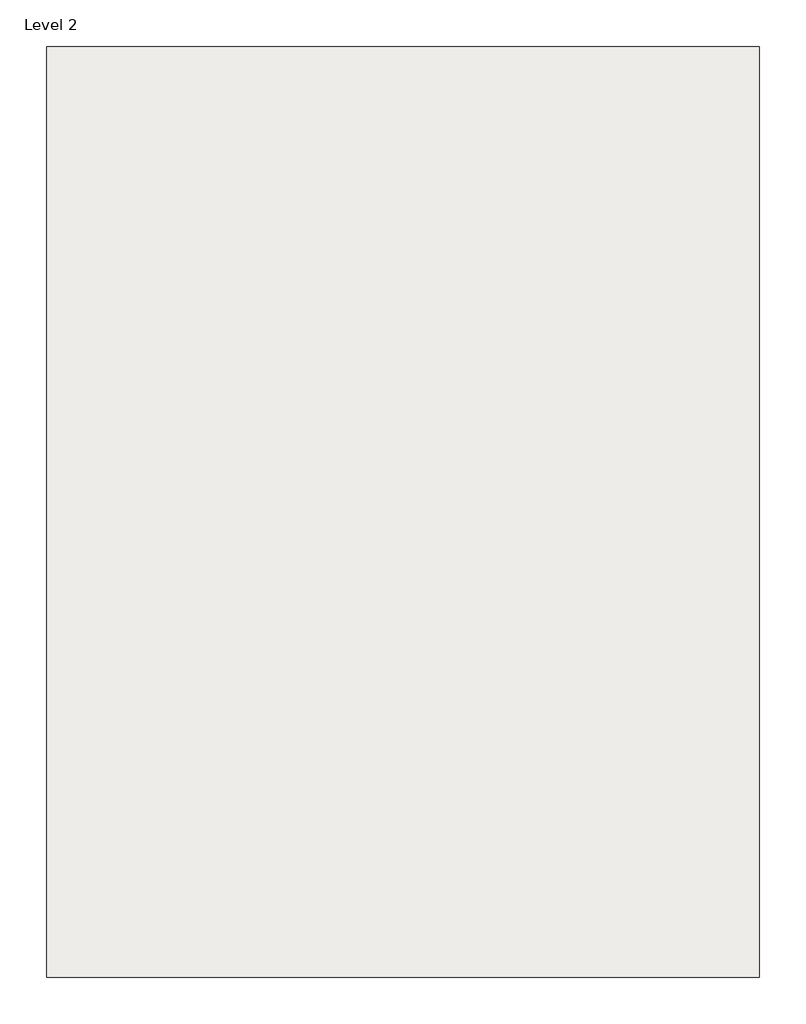
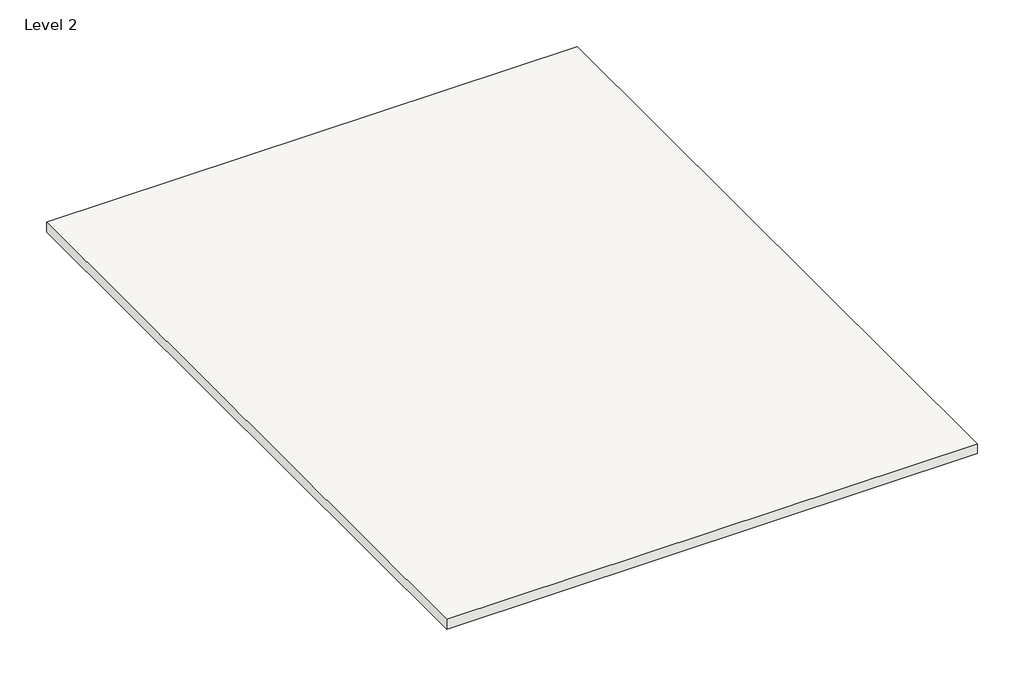
# One storey, incomplete: 1 roof.
"""IFC4 building model written with IfcOpenShell, lengths in millimetres."""

from ifc_helpers import new_model, si_unit, frame, origin, place, context, project, spatial, polyline, outline, extrude, element, save

model = new_model("IFC4")

# Units and contexts
model_context = context("Model", 3, world=origin())
ifc_project = project(units=[si_unit("LENGTHUNIT", "METRE", prefix="MILLI")], contexts=[model_context])

# Site, building, storey
site = spatial("IfcSite", under=ifc_project)
building = spatial("IfcBuilding", under=site)
storey = spatial("IfcBuildingStorey", under=building, Name="Level 2", Elevation=3048.0)

# Roof
placement = place(None, origin())
element("IfcRoof", 1, ObjectType="Generic - 12\"", at=placement, inside=storey, context=model_context, shape_type="SweptSolid", body=[
    extrude(outline(polyline([(-5198.5915084, 5688.0435985), (2688.1084916, 5688.0435985), (2688.1084916, -4611.6564015), (-5198.5915084, -4611.6564015), (-5198.5915084, 5688.0435985)])), frame((0.0, 0.0, 3048.0), z_axis=(0.0, 0.0, 1.0), x_axis=(1.0, 0.0, 0.0)), (0.0, 0.0, 1.0), 152.4),
])

save(model, "model.ifc")

# Revit data of these elements
# Type "Generic - 12\""
#   Assembly Code = "B1020"
#   Layers, outside or top first: 0' - 6" no material (function 1)
# Element 1 (IfcRoof, "Generic - 12\"")
#   built-in parameter 1001705 = 10.5 (stored number, unit not read)
#   built-in parameter 1001710 = 33615
#   Phase Created = New Construction
#   Materials on its faces: "Default Roof"
# Materials
#   "Default Roof": colour RGB 88 101 114, transparency 0, Cost = 0
